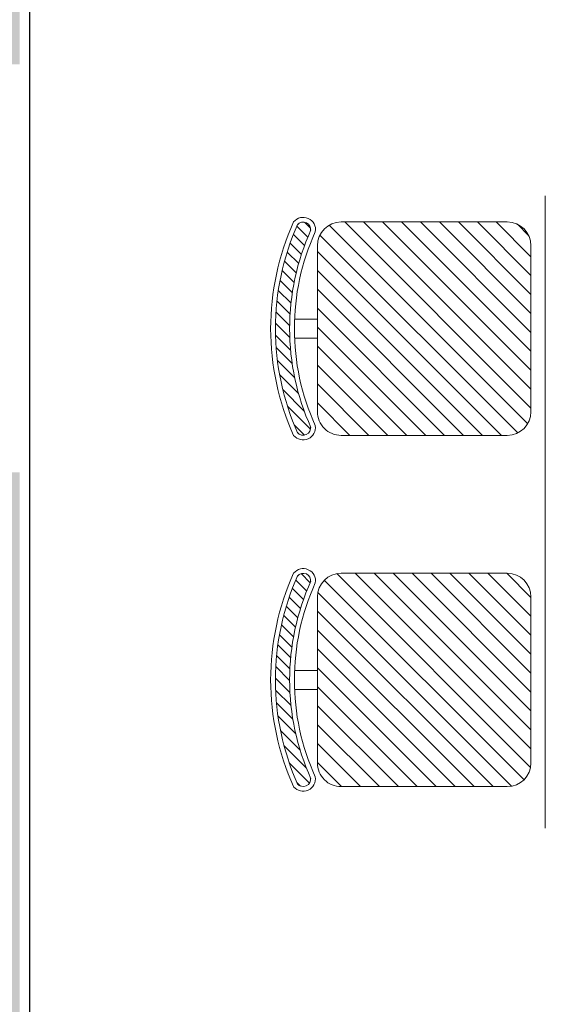
# Model space of a CAD drawing. Units: inches. Extents: x 375 to 1122, y 27 to 1069.
# Tile 8 of 155: x 667 to 705, y 253 to 326. Entities that reach past the tile are written whole.
import ezdxf

# ---------------------------------------------------------------- set-up
doc = ezdxf.new("R2010")
doc.units = ezdxf.units.IN
for name, color, linetype, lineweight in [('A-ANNO-DIMS', 2, 'Continuous', 18), ('A-COLS-PATT', 10, 'Continuous', 13), ('A-WALL-PATT', 252, 'Continuous', 13), ('Furniture', 30, 'Continuous', 18)]:
    doc.layers.add(name, color=color, linetype=linetype, lineweight=lineweight)
doc.styles.get("Standard").update_dxf_attribs({"font": 'arial.ttf'})
doc.dimstyles.new('ISO-25', dxfattribs={"dimtxt": 12, "dimasz": 2.5, "dimexe": 1.5, "dimexo": 1.5, "dimtad": 1, "dimdec": 1, "dimlunit": 3, "dimtxsty": 'Standard', "dimblk": 'ARCHTICK', "dimcen": 2.5, "dimadec": 0, "dimazin": 0, "dimtfac": 1, "dimtdec": 1, "dimtmove": 0, "dimatfit": 3, "dimfxl": 1.5, "dimfxlon": 1, "dimarcsym": 0})

# ---------------------------------------------------------------- blocks, each defined once
blk = doc.blocks.new('A$C403C54AD')
for p, q in [((0.8357, 0.5048, -0.0006), (1.9992, 0.5048, -0.0006)), ((1.2329, 0.4785, -0.0006), (0.9275, 0.4785, -0.0006)), ((1.8792, 0.4785, -0.0006), (1.5738, 0.4785, -0.0006)), ((0.8839, 0.4349, -0.0006), (0.8839, 0.304, -0.0006)), ((1.2765, 0.1295, -0.0006), (1.2765, 0.4349, -0.0006)), ((1.5302, 0.4349, -0.0006), (1.5302, 0.304, -0.0006)), ((1.9228, 0.1295, -0.0006), (1.9228, 0.4349, -0.0006)), ((0.8839, 0.304, -0.0006), (0.8839, 0.1295, -0.0006)), ((1.5302, 0.304, -0.0006), (1.5302, 0.1295, -0.0006)), ((0.9275, 0.0859, -0.0006), (1.2329, 0.0859, -0.0006)), ((1.0628, 0.0859, -0.0006), (1.0628, 0.0436, -0.0006)), ((1.0977, 0.0859, -0.0006), (1.0977, 0.0436, -0.0006)), ((1.5738, 0.0859, -0.0006), (1.8792, 0.0859, -0.0006)), ((1.7091, 0.0859, -0.0006), (1.7091, 0.0436, -0.0006)), ((1.744, 0.0859, -0.0006), (1.744, 0.0436, -0.0006))]:
    blk.add_line(p, q)
at = {"ltscale": 0.05}
for p, q in [((1.2263, 0.4785, -0.0006), (0.8839, 0.1361, -0.0006)), ((1.1915, 0.4785, -0.0006), (0.8839, 0.1709, -0.0006)), ((1.1567, 0.4785, -0.0006), (0.8839, 0.2057, -0.0006)), ((1.1218, 0.4785, -0.0006), (0.8839, 0.2406, -0.0006)), ((1.087, 0.4785, -0.0006), (0.8839, 0.2754, -0.0006)), ((1.0522, 0.4785, -0.0006), (0.8839, 0.3102, -0.0006)), ((1.0174, 0.4785, -0.0006), (0.8839, 0.3451, -0.0006)), ((0.9825, 0.4785, -0.0006), (0.8839, 0.3799, -0.0006)), ((0.9477, 0.4785, -0.0006), (0.8839, 0.4147, -0.0006)), ((0.9085, 0.4742, -0.0006), (0.8882, 0.4539, -0.0006)), ((1.2551, 0.4725, -0.0006), (0.8899, 0.1073, -0.0006)), ((1.8532, 0.4785, -0.0006), (1.5302, 0.1555, -0.0006)), ((1.8184, 0.4785, -0.0006), (1.5302, 0.1903, -0.0006)), ((1.7836, 0.4785, -0.0006), (1.5302, 0.2252, -0.0006)), ((1.7487, 0.4785, -0.0006), (1.5302, 0.26, -0.0006)), ((1.7139, 0.4785, -0.0006), (1.5302, 0.2948, -0.0006)), ((1.6791, 0.4785, -0.0006), (1.5302, 0.3296, -0.0006)), ((1.6443, 0.4785, -0.0006), (1.5302, 0.3645, -0.0006)), ((1.6094, 0.4785, -0.0006), (1.5302, 0.3993, -0.0006)), ((1.5746, 0.4785, -0.0006), (1.5302, 0.4341, -0.0006)), ((1.8873, 0.4778, -0.0006), (1.5309, 0.1214, -0.0006)), ((1.2719, 0.4545, -0.0006), (0.9079, 0.0905, -0.0006)), ((1.9101, 0.4658, -0.0006), (1.543, 0.0986, -0.0006)), ((1.9221, 0.4429, -0.0006), (1.5658, 0.0866, -0.0006)), ((1.2765, 0.4243, -0.0006), (0.9381, 0.0859, -0.0006)), ((1.9228, 0.4089, -0.0006), (1.5999, 0.0859, -0.0006)), ((1.2765, 0.3895, -0.0006), (0.973, 0.0859, -0.0006)), ((1.9228, 0.374, -0.0006), (1.6347, 0.0859, -0.0006)), ((1.2765, 0.3546, -0.0006), (1.0078, 0.0859, -0.0006)), ((1.9228, 0.3392, -0.0006), (1.6695, 0.0859, -0.0006)), ((1.2765, 0.3198, -0.0006), (1.0426, 0.0859, -0.0006)), ((1.9228, 0.3044, -0.0006), (1.7043, 0.0859, -0.0006)), ((1.2765, 0.285, -0.0006), (1.0774, 0.0859, -0.0006)), ((1.9228, 0.2695, -0.0006), (1.7392, 0.0859, -0.0006)), ((1.2765, 0.2501, -0.0006), (1.1123, 0.0859, -0.0006)), ((1.9228, 0.2347, -0.0006), (1.774, 0.0859, -0.0006)), ((1.2765, 0.2153, -0.0006), (1.1471, 0.0859, -0.0006)), ((1.9228, 0.1999, -0.0006), (1.8088, 0.0859, -0.0006)), ((1.2765, 0.1805, -0.0006), (1.1819, 0.0859, -0.0006)), ((1.9228, 0.1651, -0.0006), (1.8437, 0.0859, -0.0006)), ((1.2765, 0.1457, -0.0006), (1.2168, 0.0859, -0.0006)), ((1.9228, 0.1302, -0.0006), (1.8785, 0.0859, -0.0006)), ((0.8952, 0.0734, -0.0006), (0.8843, 0.0625, -0.0006)), ((1.2652, 0.0733, -0.0006), (1.2228, 0.0309, -0.0006)), ((1.5475, 0.0727, -0.0006), (1.5309, 0.0561, -0.0006)), ((0.9118, 0.0682, -0.0006), (0.8918, 0.0483, -0.0006)), ((0.9274, 0.0621, -0.0006), (0.9072, 0.0418, -0.0006)), ((0.9436, 0.0565, -0.0006), (0.923, 0.0359, -0.0006)), ((1.2317, 0.0616, -0.0006), (1.1924, 0.0224, -0.0006)), ((1.276, 0.0624, -0.0006), (1.2569, 0.0433, -0.0006)), ((1.5629, 0.0663, -0.0006), (1.5428, 0.0462, -0.0006)), ((1.5787, 0.0603, -0.0006), (1.5583, 0.04, -0.0006)), ((1.595, 0.0549, -0.0006), (1.5743, 0.0341, -0.0006)), ((1.8888, 0.0658, -0.0006), (1.8478, 0.0247, -0.0006)), ((1.9162, 0.0714, -0.0006), (1.8791, 0.0343, -0.0006)), ((1.9217, 0.0551, -0.0006), (1.9149, 0.0482, -0.0006)), ((0.9603, 0.0515, -0.0006), (0.9393, 0.0304, -0.0006)), ((0.9776, 0.047, -0.0006), (0.9561, 0.0255, -0.0006)), ((0.9955, 0.0431, -0.0006), (0.9734, 0.021, -0.0006)), ((1.014, 0.0399, -0.0006), (0.9914, 0.0172, -0.0006)), ((1.0333, 0.0374, -0.0006), (1.0099, 0.014, -0.0006)), ((1.1197, 0.0367, -0.0006), (1.0919, 0.0089, -0.0006)), ((1.1443, 0.0396, -0.0006), (1.1148, 0.01, -0.0006)), ((1.1708, 0.0443, -0.0006), (1.139, 0.0124, -0.0006)), ((1.1996, 0.0513, -0.0006), (1.1647, 0.0164, -0.0006)), ((1.6119, 0.05, -0.0006), (1.5907, 0.0288, -0.0006)), ((1.6293, 0.0457, -0.0006), (1.6077, 0.024, -0.0006)), ((1.6474, 0.042, -0.0006), (1.6252, 0.0198, -0.0006)), ((1.6662, 0.039, -0.0006), (1.6433, 0.0162, -0.0006)), ((1.6857, 0.0368, -0.0006), (1.6621, 0.0132, -0.0006)), ((1.7734, 0.0374, -0.0006), (1.7451, 0.0091, -0.0006)), ((1.7986, 0.0408, -0.0006), (1.7684, 0.0106, -0.0006)), ((1.8257, 0.0462, -0.0006), (1.793, 0.0135, -0.0006)), ((1.8554, 0.0541, -0.0006), (1.8193, 0.018, -0.0006)), ((1.0534, 0.0357, -0.0006), (1.0292, 0.0115, -0.0006)), ((1.0744, 0.0349, -0.0006), (1.0492, 0.0098, -0.0006)), ((1.0964, 0.0352, -0.0006), (1.0701, 0.0088, -0.0006)), ((1.7061, 0.0354, -0.0006), (1.6816, 0.0109, -0.0006)), ((1.7274, 0.0349, -0.0006), (1.7019, 0.0094, -0.0006)), ((1.7498, 0.0355, -0.0006), (1.723, 0.0087, -0.0006))]:
    blk.add_line(p, q, dxfattribs=at)
for centre, radius, start, end in [((0.9275, 0.4349, -0.0006), 0.0436, 90, 180), ((1.2329, 0.4349, -0.0006), 0.0436, 0, 90), ((1.5738, 0.4349, -0.0006), 0.0436, 90, 180), ((1.8792, 0.4349, -0.0006), 0.0436, 0, 90), ((0.9275, 0.1295, -0.0006), 0.0436, 180, 270), ((1.2329, 0.1295, -0.0006), 0.0436, 270, 0), ((1.5738, 0.1295, -0.0006), 0.0436, 180, 270), ((1.8792, 0.1295, -0.0006), 0.0436, 270, 0), ((0.8978, 0.0599, -0.0006), 0.0225, 79.7658, 231.6694), ((0.8978, 0.0599, -0.0006), 0.0138, 79.7658, 231.6694), ((1.0802, 0.4774, -0.0006), 0.4425, 245.7176, 294.2824), ((1.0802, 0.4774, -0.0006), 0.4338, 245.7176, 294.2824), ((1.2624, 0.0598, -0.0006), 0.0225, 308.8964, 99.6684), ((1.2624, 0.0598, -0.0006), 0.0138, 308.8964, 99.6684), ((1.5441, 0.0599, -0.0006), 0.0225, 79.7658, 231.6694), ((1.5441, 0.0599, -0.0006), 0.0138, 79.7658, 231.6694), ((1.7265, 0.4774, -0.0006), 0.4425, 245.7176, 294.2824), ((1.7265, 0.4774, -0.0006), 0.4338, 245.7176, 294.2824), ((1.9087, 0.0598, -0.0006), 0.0225, 308.8964, 99.6684), ((1.9087, 0.0598, -0.0006), 0.0138, 308.8964, 99.6684), ((1.0802, 0.4774, -0.0006), 0.4774, 245.7176, 294.2824), ((1.0802, 0.4774, -0.0006), 0.4687, 245.7176, 294.2824), ((1.7265, 0.4774, -0.0006), 0.4774, 245.7176, 294.2824), ((1.7265, 0.4774, -0.0006), 0.4687, 245.7176, 294.2824)]:
    blk.add_arc(centre, radius, start, end)
blk = doc.blocks.new('_ArchTick')
at = {"color": 0, "linetype": 'ByBlock', "const_width": 0.15}
blk.add_lwpolyline([(-0.5, -0.5), (0.5, 0.5)], dxfattribs=at)
blk = doc.blocks.new('*D59')
at = {"layer": 'A-ANNO-DIMS', "color": 0, "lineweight": -2, "transparency": 16777216}
for p, q in [((668.717, 346.851), (665.717, 346.851)), ((667.217, 346.851), (667.217, 232.348)), ((668.717, 232.348), (665.717, 232.348)), ((667.217, 232.348), (667.217, 27.496))]:
    blk.add_line(p, q, dxfattribs=at)
at = {"layer": 'Defpoints', "color": 0, "transparency": 16777216}
for p in [(684.392, 346.851), (667.217, 232.348), (684.392, 232.348)]:
    blk.add_point(p, dxfattribs=at)
at = {"layer": 'A-ANNO-DIMS', "color": 0, "lineweight": -2, "transparency": 16777216, "xscale": 2.5, "yscale": 2.5, "zscale": 2.5}
for p, rotation in [((667.217, 346.851), 90), ((667.217, 232.348), 270)]:
    blk.add_blockref('_ArchTick', p, dxfattribs=dict(at, rotation=rotation))
at = {"layer": 'A-ANNO-DIMS', "color": 0, "transparency": 16777216, "insert": (660.387, 128.672), "char_height": 12, "attachment_point": 5, "rotation": 90}
blk.add_mtext('DINING SET 9\'-6 1/2" TYP.', dxfattribs=at)

msp = doc.modelspace()

# ---------------------------------------------------------------- hatches: boundary and pattern name
at = {"layer": 'A-COLS-PATT'}
h = msp.add_hatch(color=256, dxfattribs=at)
h.dxf.hatch_style = 1
h.paths.add_polyline_path([(512.507, 982.528), (498.507, 982.528), (498.507, 973.528), (512.507, 973.528)])
h.paths.add_polyline_path([(666.507, 982.528), (652.507, 982.528), (652.507, 973.528), (666.507, 973.528)])
h.paths.add_polyline_path([(802.007, 982.528), (788.007, 982.528), (788.007, 973.528), (802.007, 973.528)])
h.paths.add_polyline_path([(932.007, 982.528), (918.007, 982.528), (918.007, 973.528), (932.007, 973.528)])
h.paths.add_polyline_path([(507.507, 841.528), (498.507, 841.528), (498.507, 827.528), (507.507, 827.528)])
h.paths.add_polyline_path([(666.507, 844.528), (652.507, 844.528), (652.507, 835.528), (666.507, 835.528)])
h.paths.add_polyline_path([(802.007, 814.528), (788.007, 814.528), (788.007, 805.528), (802.007, 805.528)])
h.paths.add_polyline_path([(932.007, 814.528), (918.007, 814.528), (918.007, 805.528), (932.007, 805.528)])
h.paths.add_polyline_path([(507.507, 719.528), (498.507, 719.528), (498.507, 705.528), (507.507, 705.528)])
h.paths.add_polyline_path([(731.007, 676.528), (722.007, 676.528), (722.007, 662.528), (731.007, 662.528)])
h.paths.add_polyline_path([(802.007, 676.528), (788.007, 676.528), (788.007, 667.528), (802.007, 667.528)])
h.paths.add_polyline_path([(932.007, 676.528), (918.007, 676.528), (918.007, 667.528), (932.007, 667.528)])
h.paths.add_polyline_path([(932.007, 583.528), (918.007, 583.528), (918.007, 574.528), (932.007, 574.528)])
h.paths.add_polyline_path([(868.007, 583.528), (854.007, 583.528), (854.007, 574.528), (868.007, 574.528)])
h.paths.add_polyline_path([(868.007, 502.528), (854.007, 502.528), (854.007, 493.528), (868.007, 493.528)])
h.paths.add_polyline_path([(932.007, 502.528), (918.007, 502.528), (918.007, 493.528), (932.007, 493.528)])
h.paths.add_polyline_path([(672.507, 592.028), (663.507, 592.028), (663.507, 578.028), (672.507, 578.028)])
h.paths.add_polyline_path([(512.507, 589.528), (498.507, 589.528), (498.507, 580.528), (512.507, 580.528)])
h.paths.add_polyline_path([(507.507, 464.528), (498.507, 464.528), (498.507, 450.528), (507.507, 450.528)])
h.paths.add_polyline_path([(731.007, 507.528), (722.007, 507.528), (722.007, 493.528), (731.007, 493.528)])
h.paths.add_polyline_path([(802.007, 502.528), (788.007, 502.528), (788.007, 493.528), (802.007, 493.528)])
h.paths.add_polyline_path([(507.507, 342.528), (498.507, 342.528), (498.507, 328.528), (507.507, 328.528)])
h.paths.add_polyline_path([(512.507, 196.528), (498.507, 196.528), (498.507, 187.528), (512.507, 187.528)])
h.paths.add_polyline_path([(666.507, 334.528), (652.507, 334.528), (652.507, 325.528), (666.507, 325.528)])
h.paths.add_polyline_path([(666.507, 196.528), (652.507, 196.528), (652.507, 187.528), (666.507, 187.528)])
h.paths.add_polyline_path([(805.007, 196.528), (791.007, 196.528), (791.007, 187.528), (805.007, 187.528)])
h.paths.add_polyline_path([(932.007, 196.528), (918.007, 196.528), (918.007, 187.528), (932.007, 187.528)])
h.paths.add_polyline_path([(932.007, 334.528), (918.007, 334.528), (918.007, 325.528), (932.007, 325.528)])
h.paths.add_polyline_path([(805.007, 334.528), (791.007, 334.528), (791.007, 325.528), (805.007, 325.528)])
at = {"layer": 'A-WALL-PATT'}
h = msp.add_hatch(color=256, dxfattribs=at)
h.dxf.hatch_style = 1
h.paths.add_polyline_path([(962.007, 388.528), (989.007, 388.528), (989.007, 394.528), (962.007, 394.528), (932.007, 394.528), (932.007, 397.528), (923.007, 397.528), (923.007, 394.528), (842.007, 394.528), (842.007, 334.528), (839.507, 334.528), (839.507, 328.528), (854.007, 328.528), (854.007, 334.528), (848.007, 334.528), (848.007, 388.528), (953.007, 388.528), (953.007, 356.081), (962.007, 356.081), (962.007, 358.554), (989.007, 358.554), (989.007, 364.554), (962.007, 364.554)])
h.paths.add_polyline_path([(989.007, 502.528), (932.007, 502.528), (932.007, 583.528), (932.007, 593.528), (923.007, 593.528), (923.007, 583.528), (854.007, 583.528), (854.007, 556.528), (863.007, 556.528), (863.007, 574.528), (923.007, 574.528), (923.007, 502.528), (863.007, 502.528), (863.007, 520.528), (854.007, 520.528), (854.007, 502.528), (773.007, 502.528), (773.007, 493.528), (788.007, 493.528), (788.007, 402.028), (722.007, 402.028), (722.007, 373.528), (728.007, 373.528), (728.007, 396.028), (788.007, 396.028), (788.007, 373.528), (794.007, 373.528), (794.007, 430.528), (814.007, 430.528), (814.007, 436.528), (794.007, 436.528), (794.007, 493.528), (923.007, 493.528), (923.007, 487.528), (932.007, 487.528), (932.007, 493.528), (983.007, 493.528), (983.007, 473.528), (989.007, 473.528)])
h.paths.add_polyline_path([(797.007, 325.528), (805.007, 325.528), (805.007, 328.528), (807.507, 328.528), (807.507, 334.528), (791.007, 334.528), (791.007, 226.528), (770.757, 226.528), (770.757, 217.528), (791.007, 217.528), (791.007, 187.528), (855.007, 187.528), (855.007, 196.528), (797.007, 196.528)])
h.paths.add_polyline_path([(989.007, 238.528), (962.007, 238.528), (962.007, 256.424), (953.007, 256.424), (953.007, 229.528), (980.007, 229.528), (980.007, 196.528), (915.007, 196.528), (915.007, 187.528), (989.007, 187.528)])
h.paths.add_polyline_path([(962.007, 334.528), (884.007, 334.528), (884.007, 328.528), (918.007, 328.528), (918.007, 325.528), (932.007, 325.528), (932.007, 328.528), (953.007, 328.528), (953.007, 304.424), (962.007, 304.424)])
h.paths.add_polyline_path([(606.507, 283.528), (609.507, 283.528), (609.507, 289.528), (600.507, 289.528), (600.507, 196.528), (578.507, 196.528), (578.507, 187.528), (606.507, 187.528), (606.507, 196.528)])
h.paths.add_polyline_path([(666.507, 292.528), (660.507, 292.528), (660.507, 289.528), (633.507, 289.528), (633.507, 283.528), (660.507, 283.528), (660.507, 196.528), (628.007, 196.528), (628.007, 187.528), (630.534, 187.528), (630.534, 160.528), (636.534, 160.528), (636.534, 187.528), (660.507, 187.528), (660.507, 160.528), (666.507, 160.528), (666.507, 217.528), (686.757, 217.528), (686.757, 226.528), (666.507, 226.528)])
h.paths.add_polyline_path([(480.507, 256.424), (471.507, 256.424), (471.507, 238.528), (444.507, 238.528), (444.507, 187.528), (518.507, 187.528), (518.507, 196.528), (453.507, 196.528), (453.507, 229.528), (480.507, 229.528)])
h.paths.add_polyline_path([(480.507, 328.528), (652.507, 328.528), (652.507, 325.528), (660.507, 325.528), (660.507, 322.528), (666.507, 322.528), (666.507, 334.528), (507.507, 334.528), (507.507, 360.528), (498.507, 360.528), (498.507, 334.528), (471.507, 334.528), (471.507, 304.424), (480.507, 304.424)])
h.paths.add_polyline_path([(507.507, 484.528), (498.507, 484.528), (498.507, 444.528), (507.507, 444.528), (507.507, 454.528), (621.507, 454.528), (621.507, 460.528), (507.507, 460.528)])
h.paths.add_polyline_path([(672.507, 604.528), (683.257, 604.528), (683.257, 613.528), (669.507, 613.528), (669.507, 649.528), (663.507, 649.528), (663.507, 589.528), (507.507, 589.528), (507.507, 613.528), (498.507, 613.528), (498.507, 556.528), (507.507, 556.528), (507.507, 580.528), (663.507, 580.528), (663.507, 520.528), (669.507, 520.528), (669.507, 556.528), (683.257, 556.528), (683.257, 565.528), (672.507, 565.528)])
h.paths.add_polyline_path([(731.007, 667.528), (734.007, 667.528), (734.007, 676.528), (728.007, 676.528), (728.007, 715.528), (657.507, 715.528), (657.507, 709.528), (663.507, 709.528), (663.507, 673.528), (669.507, 673.528), (669.507, 709.528), (722.007, 709.528), (722.007, 613.528), (704.757, 613.528), (704.757, 604.528), (722.007, 604.528), (722.007, 565.528), (704.757, 565.528), (704.757, 556.528), (722.007, 556.528), (722.007, 502.528), (722.007, 460.528), (669.507, 460.528), (669.507, 496.528), (663.507, 496.528), (663.507, 460.528), (657.507, 460.528), (657.507, 454.528), (728.007, 454.528), (728.007, 493.528), (734.007, 493.528), (734.007, 502.528), (731.007, 502.528)])
h.paths.add_polyline_path([(986.007, 718.528), (959.007, 718.528), (959.007, 727.528), (950.007, 727.528), (950.007, 709.528), (977.007, 709.528), (977.007, 676.528), (794.007, 676.528), (794.007, 805.528), (802.007, 805.528), (802.007, 808.528), (804.507, 808.528), (804.507, 814.528), (788.007, 814.528), (788.007, 774.028), (728.007, 774.028), (728.007, 796.528), (722.007, 796.528), (722.007, 768.028), (788.007, 768.028), (788.007, 676.528), (773.007, 676.528), (773.007, 667.528), (923.007, 667.528), (923.007, 657.528), (932.007, 657.528), (932.007, 667.528), (986.007, 667.528)])
h.paths.add_polyline_path([(621.507, 715.528), (507.507, 715.528), (507.507, 733.528), (498.507, 733.528), (498.507, 715.528), (498.507, 685.528), (507.507, 685.528), (507.507, 709.528), (621.507, 709.528)])
h.paths.add_polyline_path([(666.507, 847.028), (660.507, 847.028), (660.507, 844.528), (652.507, 844.528), (652.507, 841.528), (480.507, 841.528), (480.507, 859.528), (471.507, 859.528), (471.507, 835.528), (498.507, 835.528), (498.507, 817.528), (507.507, 817.528), (507.507, 835.528), (666.507, 835.528)])
h.paths.add_polyline_path([(480.507, 940.528), (453.507, 940.528), (453.507, 973.528), (518.507, 973.528), (518.507, 982.528), (444.507, 982.528), (444.507, 931.528), (471.507, 931.528), (471.507, 907.528), (480.507, 907.528)])
h.paths.add_polyline_path([(606.507, 982.528), (578.507, 982.528), (578.507, 973.528), (600.507, 973.528), (600.507, 880.528), (609.507, 880.528), (609.507, 886.528), (606.507, 886.528)])
h.paths.add_polyline_path([(666.507, 943.528), (686.757, 943.528), (686.757, 952.528), (666.507, 952.528), (666.507, 1009.528), (660.507, 1009.528), (660.507, 982.528), (636.534, 982.528), (636.534, 1009.528), (630.534, 1009.528), (630.534, 982.528), (628.007, 982.528), (628.007, 973.528), (660.507, 973.528), (660.507, 886.528), (633.507, 886.528), (633.507, 880.528), (660.507, 880.528), (660.507, 877.028), (666.507, 877.028)])
h.paths.add_polyline_path([(986.007, 874.528), (932.007, 874.528), (932.007, 877.528), (923.007, 877.528), (923.007, 874.528), (788.007, 874.528), (788.007, 868.528), (788.007, 844.528), (794.007, 844.528), (794.007, 868.528), (839.007, 868.528), (839.007, 814.528), (836.507, 814.528), (836.507, 808.528), (851.007, 808.528), (851.007, 814.528), (845.007, 814.528), (845.007, 868.528), (986.007, 868.528)])
h.paths.add_polyline_path([(959.007, 838.554), (986.007, 838.554), (986.007, 844.554), (959.007, 844.554), (959.007, 847.028), (950.007, 847.028), (950.007, 814.528), (881.007, 814.528), (881.007, 808.528), (918.007, 808.528), (918.007, 805.528), (932.007, 805.528), (932.007, 808.528), (950.007, 808.528), (950.007, 793.528), (959.007, 793.528)])
h.paths.add_polyline_path([(986.007, 982.528), (899.007, 982.528), (899.007, 973.528), (923.007, 973.528), (923.007, 967.528), (932.007, 967.528), (932.007, 973.528), (980.007, 973.528), (980.007, 953.528), (986.007, 953.528)])
h.paths.add_polyline_path([(851.007, 982.528), (788.007, 982.528), (788.007, 952.528), (770.757, 952.528), (770.757, 943.528), (788.007, 943.528), (788.007, 910.528), (814.007, 910.528), (814.007, 916.528), (794.007, 916.528), (794.007, 973.528), (851.007, 973.528)])

# ---------------------------------------------------------------- block references
at = {"layer": 'Furniture', "xscale": 39.9918517141215, "yscale": 39.9918517141215, "zscale": 39.9918517141215, "rotation": 270}
msp.add_blockref('A$C403C54AD', (684.955, 346.287, 0.024), dxfattribs=at)

# ---------------------------------------------------------------- dimensions: what is measured, and where the dimension line sits
at = {"layer": 'A-ANNO-DIMS'}
dim = msp.add_linear_dim(base=(667.217, 232.348), p1=(684.392, 346.851), p2=(684.392, 232.348), angle=270, text='DINING SET <> TYP.', dimstyle='ISO-25', override={"dimdec": 1, "dimlfac": 1, "dimrnd": 0, "dimzin": 1, "dimdsep": 46, "dimlunit": 4, "dimfrac": 2}, dxfattribs=at)
dim.commit()
dim.dimension.update_dxf_attribs({"geometry": '*D59', "text_midpoint": (660.387, 128.672)})

doc.saveas('drawing.dxf')
